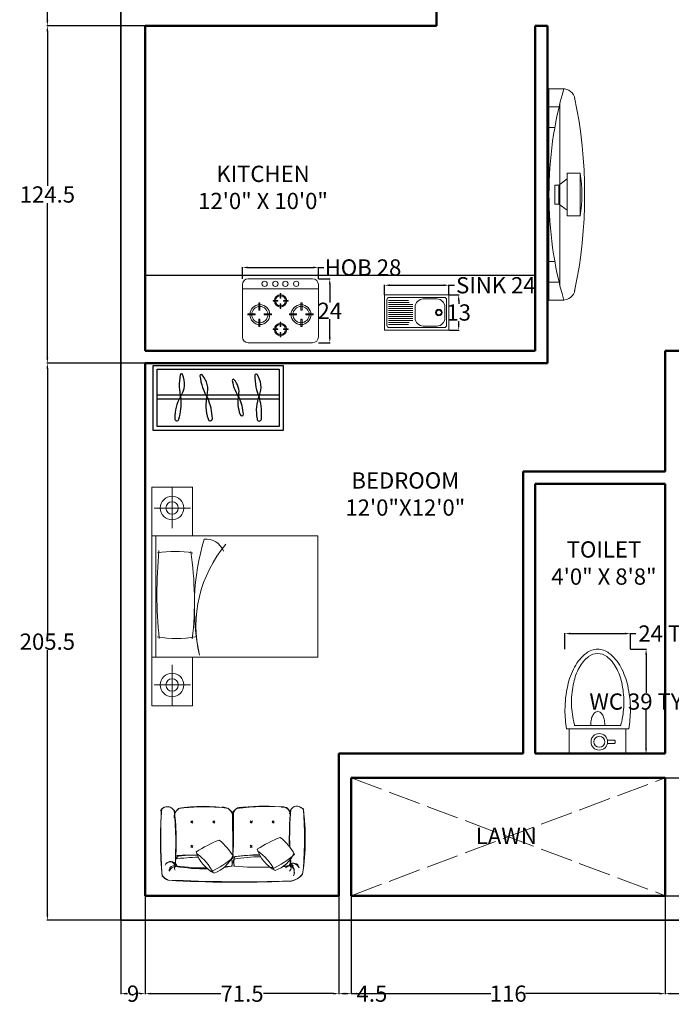
# Model space of a CAD drawing. Units: inches. Extents: x -20 to 10156, y 488 to 2970.
# Tile 1 of 6: x -20 to 221, y 488 to 851. Entities that reach past the tile are written whole.
import ezdxf

# ---------------------------------------------------------------- set-up
doc = ezdxf.new("R2010")
doc.units = ezdxf.units.IN
doc.header["$MEASUREMENT"] = 0
doc.linetypes.add('ACAD_ISO02W100', pattern=[15, 12, -3])
for name, color, linetype, lineweight in [('A-ANNO-DIMS', 2, 'Continuous', 18), ('A-AREA-IDEN', 7, 'Continuous', 25), ('A-EQPM', 9, 'Continuous', 18), ('A-FLOR-CASE', 8, 'Continuous', 25), ('A-FLOR-FIXT', 9, 'Continuous', 18), ('A-FURN', 8, 'Continuous', 18), ('A-WALL', 7, 'Continuous', 50), ('C-PROP', 7, 'Continuous', 35), ('L-PLNT-TURF', 8, 'ACAD_ISO02W100', 13)]:
    doc.layers.add(name, color=color, linetype=linetype, lineweight=lineweight)
doc.styles.get("Standard").update_dxf_attribs({"font": 'arial.ttf'})
doc.dimstyles.get("Standard").update_dxf_attribs({"dimtxt": 6, "dimasz": 2, "dimexe": 0.18, "dimexo": 0.0625, "dimgap": 0.09, "dimtad": 0, "dimtih": 1, "dimtoh": 1, "dimdec": 0, "dimzin": 0, "dimdsep": 46, "dimlunit": 4, "dimtxsty": 'Standard', "dimcen": 0.09, "dimadec": 0, "dimazin": 0, "dimtfac": 1, "dimtdec": 0, "dimtofl": 0, "dimtmove": 0, "dimatfit": 3, "dimfxl": 1, "dimtolj": 1, "dimtzin": 0, "dimarcsym": 0})

# ---------------------------------------------------------------- blocks, each defined once
blk = doc.blocks.new('A$C025C2FF6')
for p, q in [((45, 500), (550, 500)), ((0, 45), (0, 455)), ((241.9, 397.2), (241.9, 391.5)), ((277.6, 397.2), (241.9, 397.2)), ((241.9, 391.5), (277.6, 391.5)), ((277.6, 391.5), (277.6, 397.2)), ((295.2, 454.2), (300.9, 454.2)), ((295.2, 418.5), (295.2, 454.2)), ((300.9, 418.5), (295.2, 418.5)), ((300.9, 454.2), (300.9, 418.5)), ((322.1, 397.2), (357.7, 397.2)), ((322.1, 391.5), (322.1, 397.2)), ((357.7, 391.5), (322.1, 391.5)), ((357.7, 397.2), (357.7, 391.5)), ((595, 455), (595, 45)), ((128.2, 316.3), (128.2, 373.4)), ((128.2, 373.4), (137.4, 373.4)), ((137.4, 316.3), (128.2, 316.3)), ((137.4, 373.4), (137.4, 316.3)), ((295.2, 374), (295.2, 338.4)), ((300.9, 374), (295.2, 374)), ((295.2, 338.4), (300.9, 338.4)), ((300.9, 338.4), (300.9, 374)), ((467.8, 373.4), (458.7, 373.4)), ((458.7, 373.4), (458.7, 316.3)), ((458.7, 316.3), (467.8, 316.3)), ((467.8, 316.3), (467.8, 373.4)), ((100.1, 282.2), (43, 282.2)), ((43, 282.2), (43, 273.1)), ((43, 273.1), (100.1, 273.1)), ((100.1, 273.1), (100.1, 282.2)), ((128.2, 245.2), (128.2, 188.1)), ((137.4, 245.2), (128.2, 245.2)), ((137.4, 188.1), (137.4, 245.2)), ((171.3, 282.2), (228.3, 282.2)), ((171.3, 273.1), (171.3, 282.2)), ((228.3, 273.1), (171.3, 273.1)), ((228.3, 282.2), (228.3, 273.1)), ((367.8, 282.2), (367.8, 273.1)), ((424.8, 282.2), (367.8, 282.2)), ((367.8, 273.1), (424.8, 273.1)), ((424.8, 273.1), (424.8, 282.2)), ((458.7, 188.1), (458.7, 245.2)), ((458.7, 245.2), (467.8, 245.2)), ((467.8, 245.2), (467.8, 188.1)), ((496, 273.1), (496, 282.2)), ((496, 282.2), (553, 282.2)), ((553, 273.1), (496, 273.1)), ((553, 282.2), (553, 273.1)), ((128.2, 188.1), (137.4, 188.1)), ((277.6, 173.9), (241.9, 173.9)), ((241.9, 173.9), (241.9, 168.2)), ((241.9, 168.2), (277.6, 168.2)), ((277.6, 168.2), (277.6, 173.9)), ((295.2, 195.2), (295.2, 230.9)), ((295.2, 230.9), (300.9, 230.9)), ((300.9, 195.2), (295.2, 195.2)), ((300.9, 230.9), (300.9, 195.2)), ((322.1, 168.2), (322.1, 173.9)), ((322.1, 173.9), (357.7, 173.9)), ((357.7, 168.2), (322.1, 168.2)), ((357.7, 173.9), (357.7, 168.2)), ((467.8, 188.1), (458.7, 188.1)), ((300.9, 150.7), (295.2, 150.7)), ((295.2, 150.7), (295.2, 115.1)), ((295.2, 115.1), (300.9, 115.1)), ((300.9, 115.1), (300.9, 150.7)), ((1.2, 76.7), (594.9, 76.7)), ((550, 0), (45, 0))]:
    blk.add_line(p, q)
at = {"extrusion": (1e-16, 1e-16, -1)}
for centre, start_param, end_param in [((45, 455), 3.926991, 5.497787), ((550, 45), 0.785398, 2.356194)]:
    blk.add_ellipse(centre, major_axis=(31.8, 31.8), ratio=1, start_param=start_param, end_param=end_param, dxfattribs=at)
at = {"extrusion": (0, 0, -1)}
for centre, start_param, end_param in [((550, 455), 0.785398, 2.356194), ((45, 45), 3.926991, 5.497787)]:
    blk.add_ellipse(centre, major_axis=(-31.8, 31.8), ratio=1, start_param=start_param, end_param=end_param, dxfattribs=at)
at = {"extrusion": (1e-16, 3e-16, -1)}
for centre in [(298.7, 395.6), (298.7, 172.3)]:
    blk.add_ellipse(centre, major_axis=(-34.4, 34.4), ratio=1, start_param=5.497787, end_param=11.780972, dxfattribs=at)
at = {"extrusion": (1e-16, 2e-16, -1)}
for centre in [(298.7, 395.6), (298.7, 172.3)]:
    blk.add_ellipse(centre, major_axis=(-28.1, 28.1), ratio=1, start_param=5.497787, end_param=11.780972, dxfattribs=at)
at = {"extrusion": (-1e-16, -1e-16, -1)}
blk.add_ellipse((136.5, 279.7), major_axis=(-55.1, 55.1), ratio=1, start_param=5.497787, end_param=11.780972, dxfattribs=at)
at = {"extrusion": (0, -4e-16, -1)}
blk.add_ellipse((136.5, 279.7), major_axis=(-44.9, 44.9), ratio=1, start_param=5.497787, end_param=11.780972, dxfattribs=at)
for centre, major_axis, start_param, end_param in [((459.5, 279.7), (55.1, 55.1), 5.497787, 11.780972), ((459.5, 279.7), (44.9, 44.9), 5.497787, 11.780972), ((336.3, 39), (-14.8, 14.8), 3.926991, 10.210176), ((421.3, 39), (-14.8, 14.8), 3.926991, 10.210176)]:
    blk.add_ellipse(centre, major_axis=major_axis, ratio=1, start_param=start_param, end_param=end_param)
at = {"extrusion": (2e-16, -1e-16, -1)}
for centre in [(173.7, 39), (258.7, 39)]:
    blk.add_ellipse(centre, major_axis=(14.8, 14.8), ratio=1, start_param=3.926991, end_param=10.210176, dxfattribs=at)
blk = doc.blocks.new('A$C56104318')
for p, q in [((0, 0.609), (1.12, 0.609)), ((0, 0.609), (0, 0)), ((0.042, 0.525), (0.042, 0.084)), ((0.42, 0.515), (0.07, 0.515)), ((0.084, 0.567), (1.036, 0.567)), ((0.672, 0.539), (0.91, 0.539)), ((1.078, 0.525), (1.078, 0.084)), ((1.12, 0.609), (1.12, 0)), ((0.07, 0.48), (0.429, 0.48)), ((0.07, 0.445), (0.49, 0.445)), ((0.07, 0.41), (0.49, 0.41)), ((0.07, 0.375), (0.49, 0.375)), ((0.532, 0.21), (0.532, 0.399)), ((1.05, 0.399), (1.05, 0.21)), ((0.07, 0.34), (0.49, 0.34)), ((0.07, 0.305), (0.49, 0.305)), ((0.07, 0.27), (0.49, 0.27)), ((0.07, 0.235), (0.49, 0.235)), ((0.07, 0.2), (0.49, 0.2)), ((0.07, 0.165), (0.49, 0.165)), ((0.07, 0.13), (0.429, 0.13)), ((0.07, 0.094), (0.42, 0.094)), ((1.036, 0.042), (0.084, 0.042)), ((0.91, 0.07), (0.672, 0.07)), ((1.12, 0), (0, 0))]:
    blk.add_line(p, q)
for radius in [0.0574, 0.0427]:
    blk.add_circle((0.945, 0.305), radius)
for centre, radius, start, end in [((0.084, 0.525), 0.042, 90, 180), ((0.672, 0.399), 0.14, 90, 180), ((0.91, 0.399), 0.14, 0, 90), ((1.036, 0.525), 0.042, 0, 90), ((0.672, 0.21), 0.14, 180, 270), ((0.91, 0.21), 0.14, 270, 0), ((0.084, 0.084), 0.042, 180, 270), ((1.036, 0.084), 0.042, 270, 0)]:
    blk.add_arc(centre, radius, start, end)
blk = doc.blocks.new('A$C559B0E78')
at = {"xscale": 729, "yscale": 729, "zscale": 729}
blk.add_blockref('A$C56104318', (0, 0), dxfattribs=at)
blk = doc.blocks.new('A$C041817D3')
for p, q in [((0, 0), (0, 500)), ((0, 500), (1000, 500)), ((30, 30), (30, 470)), ((30, 470), (970, 470)), ((970, 470), (970, 30)), ((1000, 500), (1000, 0)), ((206.7, 270.8), (29.8, 270.8)), ((199, 240.8), (29.8, 240.8)), ((408.8, 240.8), (212.6, 240.8)), ((405.5, 270.8), (216.1, 270.8)), ((647.4, 270.8), (415.1, 270.8)), ((652.4, 240.8), (422, 240.8)), ((807.7, 270.8), (657.5, 270.8)), ((806.2, 240.8), (664.7, 240.8)), ((970.2, 270.8), (817, 270.8)), ((970.2, 240.8), (819.2, 240.8)), ((970, 30), (30, 30)), ((1000, 0), (0, 0))]:
    blk.add_line(p, q)
for centre, radius, start, end in [((621.4, 345.7), 421.4, 168.77299, 193.85802), ((217.3, 425.9), 9.38, 24.60956, 168.77299), ((72.1, 359.4), 169.1, 323.97798, 24.60956), ((368.6, 419.8), 9.38, 42.60956, 186.77299), ((777.7, 468.4), 421.4, 186.77299, 211.85802), ((251, 311.7), 169.1, 345.54145, 42.60956), ((615.5, 385.7), 7.5, 44.60956, 188.77299), ((941.3, 435.9), 337.1, 188.77299, 213.85802), ((524.6, 295.9), 135.3, 347.54145, 44.60956), ((791.5, 424.4), 9.38, 34.60956, 178.77299), ((1203.4, 415.6), 421.4, 178.77299, 203.85802), ((660.1, 333.7), 169.1, 337.54145, 34.60956), ((476.4, 102.2), 310, 149.58385, 181.67451), ((-230.1, 204), 444.3, 344.57561, 5.26247), ((715, 192.1), 310, 165.54145, 199.67451), ((11.6, 70.6), 444.3, 2.57561, 23.26247), ((898.8, 213.2), 248, 167.54145, 201.67451), ((339.9, 96.4), 355.4, 4.57561, 25.26247), ((1102.9, 150.7), 310, 157.54145, 191.67451), ((389.5, 128.2), 444.3, 354.57561, 15.26247), ((182.5, 90.2), 16.3, 169.40186, 344.57561), ((439.2, 89.8), 16.3, 187.40186, 2.57561), ((681.2, 123.8), 13, 189.40186, 4.57561), ((815.5, 87.8), 16.3, 179.40186, 354.57561)]:
    blk.add_arc(centre, radius, start, end)
blk = doc.blocks.new('A$C7FD35E1A')
for p, q in [((0.0233, 0.5799), (0.0233, 0.4408)), ((0.0233, 0.5799), (0.338, 0.5799)), ((0.338, 0.5799), (0.338, 0.4408)), ((0.2356, 0.5044), (0.275, 0.5044)), ((0.2357, 0.5217), (0.2745, 0.5217)), ((0.3542, 0.4408), (0.0087, 0.4408)), ((0.3093, 0.4224), (0.0536, 0.4224))]:
    blk.add_line(p, q)
for radius in [0.046, 0.0305]:
    blk.add_circle((0.1904, 0.5132), radius)
for centre, radius, start, end in [((0.2685, 0.5129), 0.0107, 307.488, 55.394), ((0.6238, 0.337), 0.6238, 170.4184, 180), ((-0.261, 0.337), 0.6238, 0, 9.5816), ((0.5354, 0.2931), 0.4991, 167.4267, 180), ((0.3603, 0.3321), 0.3197, 163.5954, 167.4267), ((0.277, 0.4171), 0.1337, 177.7133, 180), ((0.277, 0.4171), 0.1337, 180, 192.5399), ((0.23, 0.4066), 0.0855, 192.5399, 208.2349), ((0.1339, 0.4066), 0.0855, 331.7651, 347.4601), ((0.0869, 0.4171), 0.1337, 347.4601, 0), ((0.0869, 0.4171), 0.1337, 360, 2.2867), ((0.0026, 0.3321), 0.3197, 12.5733, 16.4046), ((-0.1725, 0.2931), 0.4991, 0, 12.5733), ((0.6238, 0.337), 0.6238, 180, 192.5733), ((0.2004, 0.3907), 0.052, 208.2349, 232.3543), ((0.182, 0.3668), 0.0218, 232.3543, 270), ((0.182, 0.3668), 0.0218, 270, 307.6457), ((0.1635, 0.3907), 0.052, 307.6457, 331.7651), ((-0.261, 0.337), 0.6238, 347.4267, 0), ((0.5354, 0.2931), 0.4991, 180, 192.5733), ((-0.1725, 0.2931), 0.4991, 347.4267, 0), ((0.405, 0.2881), 0.3996, 192.5733, 208.3008), ((0.3603, 0.254), 0.3197, 192.5733, 208.3008), ((0.0026, 0.254), 0.3197, 331.6992, 347.4267), ((-0.0421, 0.2881), 0.3996, 331.6992, 347.4267), ((0.2672, 0.214), 0.2432, 208.3008, 232.4306), ((0.2501, 0.1947), 0.1945, 208.3008, 232.4306), ((0.1128, 0.1947), 0.1945, 307.5694, 331.6992), ((0.0957, 0.214), 0.2432, 307.5694, 331.6992), ((0.1814, 0.1024), 0.1024, 232.4306, 270), ((0.1814, 0.1055), 0.082, 232.4306, 270), ((0.1814, 0.1055), 0.082, 270, 307.5694), ((0.1814, 0.1024), 0.1024, 270, 307.5694)]:
    blk.add_arc(centre, radius, start, end)
blk = doc.blocks.new('BED-WITH-NIGHTSTANDS')
for p, q in [((0, 80.86), (14.96, 80.86)), ((0, 62.91), (0, 80.86)), ((7.48, 73.12), (7.48, 80.95)), ((14.96, 80.86), (14.96, 62.91)), ((7.48, 73.12), (0.91, 73.12)), ((7.48, 73.12), (7.48, 65.64)), ((7.48, 73.12), (14.3, 73.12)), ((0, 62.91), (13.46, 62.91)), ((61.33, 62.91), (0, 62.91)), ((0, 18.04), (0, 62.91)), ((14.96, 62.91), (0, 62.91)), ((1.5, 18.04), (1.5, 62.91)), ((61.33, 18.04), (61.33, 62.91)), ((0, 18.04), (13.46, 18.04)), ((0, 18.04), (13.46, 18.04)), ((61.33, 18.04), (0, 18.04)), ((14.96, 18.04), (0, 18.04)), ((0, 18.04), (0, 0.09)), ((7.48, 7.83), (7.48, 15.31)), ((14.96, 0.09), (14.96, 18.04)), ((7.48, 7.83), (0.91, 7.83)), ((7.48, 7.83), (7.48, 0)), ((7.48, 7.83), (14.3, 7.83)), ((0, 0.09), (14.96, 0.09))]:
    blk.add_line(p, q)
for centre, radius in [((7.48, 73.12), 4.35), ((7.48, 73.12), 2.3), ((7.48, 7.83), 4.35), ((7.48, 7.83), 2.3)]:
    blk.add_circle(centre, radius)
for centre, radius, start, end in [((104.1, 36.77), 88.38, 163.6527, 191.7538), ((62.88, 29.59), 46.58, 139.6764, 193.4364), ((19.88, 54.53), 7.14, 22.4412, 94.6731), ((161.95, 41.88), 160.07, 174.4374, 186.047), ((8.44, 20.88), 36.25, 79.3149, 100.0855), ((-111.82, 38.85), 127.54, 353.7104, 8.2351), ((8.92, 63.63), 38.69, 259.7294, 280.8239)]:
    blk.add_arc(centre, radius, start, end)
blk = doc.blocks.new('*D14')
at = {"layer": 'A-ANNO-DIMS', "color": 0, "lineweight": -2, "transparency": 16777216}
for p, q in [((206, 618.67), (211.91, 618.67)), ((211.73, 616.67), (211.73, 602.56)), ((211.73, 582.06), (211.73, 596.17)), ((206, 580.06), (211.91, 580.06))]:
    blk.add_line(p, q, dxfattribs=at)
at = {"layer": 'A-ANNO-DIMS', "color": 0, "transparency": 16777216}
for points in [[(211.4, 616.67), (212.07, 616.67), (211.73, 618.67)], [(211.4, 582.06), (212.07, 582.06), (211.73, 580.06)]]:
    blk.add_solid(points, dxfattribs=at)
at = {"layer": 'Defpoints', "color": 0, "transparency": 16777216}
for p in [(205.94, 618.67), (205.94, 580.06), (211.73, 580.06)]:
    blk.add_point(p, dxfattribs=at)
at = {"layer": 'A-ANNO-DIMS', "color": 0, "transparency": 16777216, "insert": (211.73, 599.36), "char_height": 6, "attachment_point": 5}
blk.add_mtext('\\A1;WC 39 TYP.', dxfattribs=at)
blk = doc.blocks.new('*D15')
at = {"layer": 'A-ANNO-DIMS', "color": 0, "lineweight": -2, "transparency": 16777216}
for p, q in [((181.78, 618.73), (181.78, 624.64)), ((183.78, 624.46), (203.94, 624.46)), ((205.94, 618.73), (205.94, 624.64)), ((205.94, 624.46), (207.94, 624.46))]:
    blk.add_line(p, q, dxfattribs=at)
at = {"layer": 'A-ANNO-DIMS', "color": 0, "transparency": 16777216}
for points in [[(183.78, 624.79), (183.78, 624.13), (181.78, 624.46)], [(203.94, 624.79), (203.94, 624.13), (205.94, 624.46)]]:
    blk.add_solid(points, dxfattribs=at)
at = {"layer": 'Defpoints', "color": 0, "transparency": 16777216}
for p in [(205.94, 624.46), (181.78, 618.67), (205.94, 618.67)]:
    blk.add_point(p, dxfattribs=at)
at = {"layer": 'A-ANNO-DIMS', "color": 0, "transparency": 16777216, "insert": (222.69, 624.46), "char_height": 6, "attachment_point": 5}
blk.add_mtext('\\A1;24 TYP.', dxfattribs=at)
blk = doc.blocks.new('*D24')
at = {"layer": 'A-ANNO-DIMS', "color": 0, "lineweight": -2, "transparency": 16777216}
for p, q in [((62.67, 755.4), (62.67, 759.72)), ((64.67, 759.54), (88.72, 759.54)), ((90.72, 755.4), (90.72, 759.72)), ((90.72, 759.54), (92.72, 759.54))]:
    blk.add_line(p, q, dxfattribs=at)
at = {"layer": 'A-ANNO-DIMS', "color": 0, "transparency": 16777216}
for points in [[(64.67, 759.88), (64.67, 759.21), (62.67, 759.54)], [(88.72, 759.88), (88.72, 759.21), (90.72, 759.54)]]:
    blk.add_solid(points, dxfattribs=at)
at = {"layer": 'Defpoints', "color": 0, "transparency": 16777216}
for p in [(90.72, 759.54), (62.67, 755.34), (90.72, 755.34)]:
    blk.add_point(p, dxfattribs=at)
at = {"layer": 'A-ANNO-DIMS', "color": 0, "transparency": 16777216, "insert": (107.2, 759.54), "char_height": 6, "attachment_point": 5}
blk.add_mtext('\\A1;HOB 28', dxfattribs=at)
blk = doc.blocks.new('*D25')
at = {"layer": 'A-ANNO-DIMS', "color": 0, "lineweight": -2, "transparency": 16777216}
for p, q in [((90.78, 755.34), (95.11, 755.34)), ((94.93, 753.34), (94.93, 746.65)), ((94.93, 733.76), (94.93, 740.45)), ((90.78, 731.76), (95.11, 731.76))]:
    blk.add_line(p, q, dxfattribs=at)
at = {"layer": 'A-ANNO-DIMS', "color": 0, "transparency": 16777216}
for points in [[(94.6, 753.34), (95.26, 753.34), (94.93, 755.34)], [(94.6, 733.76), (95.26, 733.76), (94.93, 731.76)]]:
    blk.add_solid(points, dxfattribs=at)
at = {"layer": 'Defpoints', "color": 0, "transparency": 16777216}
for p in [(90.72, 755.34), (90.72, 731.76), (94.93, 731.76)]:
    blk.add_point(p, dxfattribs=at)
at = {"layer": 'A-ANNO-DIMS', "color": 0, "transparency": 16777216, "insert": (94.93, 743.55), "char_height": 6, "attachment_point": 5}
blk.add_mtext('\\A1;24', dxfattribs=at)
blk = doc.blocks.new('*D26')
at = {"layer": 'A-ANNO-DIMS', "color": 0, "lineweight": -2, "transparency": 16777216}
for p, q in [((115.12, 749.47), (115.12, 753.17)), ((117.12, 752.99), (136.95, 752.99)), ((138.95, 749.47), (138.95, 753.17)), ((138.95, 752.99), (140.95, 752.99))]:
    blk.add_line(p, q, dxfattribs=at)
at = {"layer": 'A-ANNO-DIMS', "color": 0, "transparency": 16777216}
for points in [[(117.12, 753.32), (117.12, 752.65), (115.12, 752.99)], [(136.95, 753.32), (136.95, 752.65), (138.95, 752.99)]]:
    blk.add_solid(points, dxfattribs=at)
at = {"layer": 'Defpoints', "color": 0, "transparency": 16777216}
for p in [(138.95, 752.99), (115.12, 749.41), (138.95, 749.41)]:
    blk.add_point(p, dxfattribs=at)
at = {"layer": 'A-ANNO-DIMS', "color": 0, "transparency": 16777216, "insert": (156.26, 752.99), "char_height": 6, "attachment_point": 5}
blk.add_mtext('\\A1;SINK 24', dxfattribs=at)
blk = doc.blocks.new('*D27')
at = {"layer": 'A-ANNO-DIMS', "color": 0, "lineweight": -2, "transparency": 16777216}
for p, q in [((139.02, 749.41), (142.71, 749.41)), ((142.53, 747.41), (142.53, 746.09)), ((142.53, 738.45), (142.53, 739.77)), ((139.02, 736.45), (142.71, 736.45))]:
    blk.add_line(p, q, dxfattribs=at)
at = {"layer": 'A-ANNO-DIMS', "color": 0, "transparency": 16777216}
for points in [[(142.2, 747.41), (142.86, 747.41), (142.53, 749.41)], [(142.2, 738.45), (142.86, 738.45), (142.53, 736.45)]]:
    blk.add_solid(points, dxfattribs=at)
at = {"layer": 'Defpoints', "color": 0, "transparency": 16777216}
for p in [(138.95, 749.41), (138.95, 736.45), (142.53, 736.45)]:
    blk.add_point(p, dxfattribs=at)
at = {"layer": 'A-ANNO-DIMS', "color": 0, "transparency": 16777216, "insert": (142.53, 742.93), "char_height": 6, "attachment_point": 5}
blk.add_mtext('\\A1;13', dxfattribs=at)
blk = doc.blocks.new('*D32')
at = {"layer": 'A-ANNO-DIMS', "color": 0, "lineweight": -2, "transparency": 16777216}
for p, q in [((26.74, 917.23), (-9.53, 917.23)), ((-9.35, 915.23), (-9.35, 886.13)), ((-9.35, 850.73), (-9.35, 879.83)), ((26.74, 848.73), (-9.53, 848.73))]:
    blk.add_line(p, q, dxfattribs=at)
at = {"layer": 'A-ANNO-DIMS', "color": 0, "transparency": 16777216}
for points in [[(-9.68, 915.23), (-9.02, 915.23), (-9.35, 917.23)], [(-9.68, 850.73), (-9.02, 850.73), (-9.35, 848.73)]]:
    blk.add_solid(points, dxfattribs=at)
at = {"layer": 'Defpoints', "color": 0, "transparency": 16777216}
for p in [(26.8, 917.23), (-9.35, 848.73), (26.8, 848.73)]:
    blk.add_point(p, dxfattribs=at)
at = {"layer": 'A-ANNO-DIMS', "color": 0, "transparency": 16777216, "insert": (-9.35, 882.98), "char_height": 6, "attachment_point": 5}
blk.add_mtext('\\A1;68.5', dxfattribs=at)
blk = doc.blocks.new('*D33')
at = {"layer": 'A-ANNO-DIMS', "color": 0, "lineweight": -2, "transparency": 16777216}
for p, q in [((26.74, 848.73), (-9.53, 848.73)), ((-9.35, 846.73), (-9.35, 789.63)), ((-9.35, 726.23), (-9.35, 783.33)), ((26.74, 724.23), (-9.53, 724.23))]:
    blk.add_line(p, q, dxfattribs=at)
at = {"layer": 'A-ANNO-DIMS', "color": 0, "transparency": 16777216}
for points in [[(-9.68, 846.73), (-9.02, 846.73), (-9.35, 848.73)], [(-9.68, 726.23), (-9.02, 726.23), (-9.35, 724.23)]]:
    blk.add_solid(points, dxfattribs=at)
at = {"layer": 'Defpoints', "color": 0, "transparency": 16777216}
for p in [(26.8, 848.73), (-9.35, 724.23), (26.8, 724.23)]:
    blk.add_point(p, dxfattribs=at)
at = {"layer": 'A-ANNO-DIMS', "color": 0, "transparency": 16777216, "insert": (-9.35, 786.48), "char_height": 6, "attachment_point": 5}
blk.add_mtext('\\A1;124.5', dxfattribs=at)
blk = doc.blocks.new('*D34')
at = {"layer": 'A-ANNO-DIMS', "color": 0, "lineweight": -2, "transparency": 16777216}
for p, q in [((26.74, 724.23), (-9.53, 724.23)), ((-9.35, 722.23), (-9.35, 624.63)), ((-9.35, 520.73), (-9.35, 618.33)), ((17.74, 518.73), (-9.53, 518.73))]:
    blk.add_line(p, q, dxfattribs=at)
at = {"layer": 'A-ANNO-DIMS', "color": 0, "transparency": 16777216}
for points in [[(-9.68, 722.23), (-9.02, 722.23), (-9.35, 724.23)], [(-9.68, 520.73), (-9.02, 520.73), (-9.35, 518.73)]]:
    blk.add_solid(points, dxfattribs=at)
at = {"layer": 'Defpoints', "color": 0, "transparency": 16777216}
for p in [(26.8, 724.23), (-9.35, 518.73), (17.8, 518.73)]:
    blk.add_point(p, dxfattribs=at)
at = {"layer": 'A-ANNO-DIMS', "color": 0, "transparency": 16777216, "insert": (-9.35, 621.48), "char_height": 6, "attachment_point": 5}
blk.add_mtext('\\A1;205.5', dxfattribs=at)
blk = doc.blocks.new('*D35')
at = {"layer": 'A-ANNO-DIMS', "color": 0, "lineweight": -2, "transparency": 16777216}
for p, q in [((26.8, 527.67), (26.8, 491.4)), ((17.8, 518.67), (17.8, 491.4)), ((19.8, 491.58), (20.24, 491.58)), ((24.8, 491.58), (24.36, 491.58))]:
    blk.add_line(p, q, dxfattribs=at)
at = {"layer": 'A-ANNO-DIMS', "color": 0, "transparency": 16777216}
for points in [[(19.8, 491.91), (19.8, 491.25), (17.8, 491.58)], [(24.8, 491.91), (24.8, 491.25), (26.8, 491.58)]]:
    blk.add_solid(points, dxfattribs=at)
at = {"layer": 'Defpoints', "color": 0, "transparency": 16777216}
for p in [(26.8, 527.73), (17.8, 518.73), (26.8, 491.58)]:
    blk.add_point(p, dxfattribs=at)
at = {"layer": 'A-ANNO-DIMS', "color": 0, "transparency": 16777216, "insert": (22.3, 491.58), "char_height": 6, "attachment_point": 5}
blk.add_mtext('\\A1;9', dxfattribs=at)
blk = doc.blocks.new('*D36')
at = {"layer": 'A-ANNO-DIMS', "color": 0, "lineweight": -2, "transparency": 16777216}
for p, q in [((26.8, 527.67), (26.8, 491.4)), ((98.3, 527.67), (98.3, 491.4)), ((28.8, 491.58), (54.67, 491.58)), ((96.3, 491.58), (70.43, 491.58))]:
    blk.add_line(p, q, dxfattribs=at)
at = {"layer": 'A-ANNO-DIMS', "color": 0, "transparency": 16777216}
for points in [[(28.8, 491.91), (28.8, 491.25), (26.8, 491.58)], [(96.3, 491.91), (96.3, 491.25), (98.3, 491.58)]]:
    blk.add_solid(points, dxfattribs=at)
at = {"layer": 'Defpoints', "color": 0, "transparency": 16777216}
for p in [(26.8, 527.73), (98.3, 527.73), (98.3, 491.58)]:
    blk.add_point(p, dxfattribs=at)
at = {"layer": 'A-ANNO-DIMS', "color": 0, "transparency": 16777216, "insert": (62.55, 491.58), "char_height": 6, "attachment_point": 5}
blk.add_mtext('\\A1;71.5', dxfattribs=at)
blk = doc.blocks.new('*D37')
at = {"layer": 'A-ANNO-DIMS', "color": 0, "lineweight": -2, "transparency": 16777216}
for p, q in [((98.3, 527.67), (98.3, 491.4)), ((102.8, 527.67), (102.8, 491.4)), ((100.3, 491.58), (100.8, 491.58)), ((102.8, 491.58), (104.8, 491.58))]:
    blk.add_line(p, q, dxfattribs=at)
at = {"layer": 'A-ANNO-DIMS', "color": 0, "transparency": 16777216}
for points in [[(100.3, 491.91), (100.3, 491.25), (98.3, 491.58)], [(100.8, 491.91), (100.8, 491.25), (102.8, 491.58)]]:
    blk.add_solid(points, dxfattribs=at)
at = {"layer": 'Defpoints', "color": 0, "transparency": 16777216}
for p in [(98.3, 527.73), (102.8, 527.73), (102.8, 491.58)]:
    blk.add_point(p, dxfattribs=at)
at = {"layer": 'A-ANNO-DIMS', "color": 0, "transparency": 16777216, "insert": (110.49, 491.58), "char_height": 6, "attachment_point": 5}
blk.add_mtext('\\A1;4.5', dxfattribs=at)
blk = doc.blocks.new('*D38')
at = {"layer": 'A-ANNO-DIMS', "color": 0, "lineweight": -2, "transparency": 16777216}
for p, q in [((102.8, 527.67), (102.8, 491.4)), ((218.8, 527.67), (218.8, 491.4)), ((104.8, 491.58), (154.37, 491.58)), ((216.8, 491.58), (167.23, 491.58))]:
    blk.add_line(p, q, dxfattribs=at)
at = {"layer": 'A-ANNO-DIMS', "color": 0, "transparency": 16777216}
for points in [[(104.8, 491.91), (104.8, 491.25), (102.8, 491.58)], [(216.8, 491.91), (216.8, 491.25), (218.8, 491.58)]]:
    blk.add_solid(points, dxfattribs=at)
at = {"layer": 'Defpoints', "color": 0, "transparency": 16777216}
for p in [(102.8, 527.73), (218.8, 527.73), (218.8, 491.58)]:
    blk.add_point(p, dxfattribs=at)
at = {"layer": 'A-ANNO-DIMS', "color": 0, "transparency": 16777216, "insert": (160.8, 491.58), "char_height": 6, "attachment_point": 5}
blk.add_mtext('\\A1;116', dxfattribs=at)
blk = doc.blocks.new('*D39')
at = {"layer": 'A-ANNO-DIMS', "color": 0, "lineweight": -2, "transparency": 16777216}
for p, q in [((218.8, 527.67), (218.8, 491.4)), ((377.8, 518.67), (377.8, 491.4)), ((220.8, 491.58), (291.86, 491.58)), ((375.8, 491.58), (304.74, 491.58))]:
    blk.add_line(p, q, dxfattribs=at)
at = {"layer": 'A-ANNO-DIMS', "color": 0, "transparency": 16777216}
for points in [[(220.8, 491.91), (220.8, 491.25), (218.8, 491.58)], [(375.8, 491.91), (375.8, 491.25), (377.8, 491.58)]]:
    blk.add_solid(points, dxfattribs=at)
at = {"layer": 'Defpoints', "color": 0, "transparency": 16777216}
for p in [(218.8, 527.73), (377.8, 518.73), (377.8, 491.58)]:
    blk.add_point(p, dxfattribs=at)
at = {"layer": 'A-ANNO-DIMS', "color": 0, "transparency": 16777216, "insert": (298.3, 491.58), "char_height": 6, "attachment_point": 5}
blk.add_mtext('\\A1;159', dxfattribs=at)
blk = doc.blocks.new('*D40')
at = {"layer": 'A-ANNO-DIMS', "color": 0, "lineweight": -2, "transparency": 16777216}
for p, q in [((218.86, 571.23), (246.13, 571.23)), ((245.95, 569.23), (245.95, 552.64)), ((245.95, 529.73), (245.95, 546.32)), ((218.86, 527.73), (246.13, 527.73))]:
    blk.add_line(p, q, dxfattribs=at)
at = {"layer": 'A-ANNO-DIMS', "color": 0, "transparency": 16777216}
for points in [[(245.62, 569.23), (246.28, 569.23), (245.95, 571.23)], [(245.62, 529.73), (246.28, 529.73), (245.95, 527.73)]]:
    blk.add_solid(points, dxfattribs=at)
at = {"layer": 'Defpoints', "color": 0, "transparency": 16777216}
for p in [(218.8, 571.23), (218.8, 527.73), (245.95, 527.73)]:
    blk.add_point(p, dxfattribs=at)
at = {"layer": 'A-ANNO-DIMS', "color": 0, "transparency": 16777216, "insert": (245.95, 549.48), "char_height": 6, "attachment_point": 5}
blk.add_mtext('\\A1;43.5', dxfattribs=at)

msp = doc.modelspace()

# ---------------------------------------------------------------- linework, layer by layer
at = {"layer": 'A-EQPM'}
for p, q in [((175.86, 747.52), (175.86, 825.47)), ((181.35, 825.47), (175.86, 825.47)), ((181.35, 825.47), (181.39, 825.47)), ((175.86, 818.88), (179.63, 818.88)), ((179.9, 819.98), (179.9, 753.01)), ((175.86, 811.2), (178.04, 811.2)), ((182.59, 792.2), (179.55, 789.95)), ((182.59, 794.37), (187.37, 794.37)), ((182.59, 794.37), (182.59, 778.54)), ((187.37, 794.37), (187.37, 778.54)), ((178.01, 782.95), (178.01, 789.95)), ((179.55, 789.95), (178.01, 789.95)), ((179.55, 782.95), (179.55, 789.95)), ((179.55, 782.95), (178.01, 782.95)), ((182.59, 780.71), (179.55, 782.95)), ((182.59, 778.54), (187.37, 778.54)), ((175.86, 761.79), (178.04, 761.79)), ((175.86, 754.11), (179.63, 754.11)), ((175.86, 747.52), (181.35, 747.52)), ((181.35, 747.52), (181.39, 747.52))]:
    msp.add_line(p, q, dxfattribs=at)
msp.add_lwpolyline([(185.35, 822.22, -0.103184), (185.35, 750.77, -0.103184)], format="xyb", dxfattribs=at)
for centre, radius, start, end in [((316.97, 786.49), 141.11, 163.9658, 196.0342), ((181.11, 821.09), 4.39, 8.4687, 93.693), ((139.09, 786.45), 48.93, 350.6925, 9.3075), ((181.11, 751.9), 4.39, 266.307, 351.5313)]:
    msp.add_arc(centre, radius, start, end, dxfattribs=at)
at = {"layer": 'A-FLOR-CASE'}
msp.add_line((26.8, 756.73), (170.8, 756.73), dxfattribs=at)
at = {"layer": 'A-FURN'}
for p, q in [((44.41, 555.29), (43.65, 554.55)), ((43.66, 555.3), (44.4, 554.54)), ((52.51, 555.29), (51.75, 554.55)), ((51.76, 555.3), (52.5, 554.54)), ((66.34, 555.29), (65.58, 554.55)), ((65.59, 555.3), (66.33, 554.54)), ((74.43, 555.29), (73.67, 554.55)), ((73.68, 555.3), (74.42, 554.54)), ((44.37, 546.3), (43.61, 545.55)), ((43.62, 546.31), (44.36, 545.55)), ((66.3, 546.3), (65.54, 545.55)), ((65.55, 546.31), (66.29, 545.55))]:
    msp.add_line(p, q, dxfattribs=at)
for centre, radius, start, end in [((34.94, 557.78), 2.83, 14.6379, 154.3095), ((176.69, 548.41), 144.28, 175.4325, 185.431), ((244.3, 549.68), 211.76, 177.3143, 183.933), ((34.94, 557.51), 3.02, 33.041, 136.0653), ((40.96, 556.8), 3.46, 100.9756, 184.9747), ((40.86, 557.12), 3.21, 109.8228, 182.4985), ((48.43, 508), 52.71, 80.0543, 100.4167), ((48.36, 490.17), 70.37, 85.2072, 97.551), ((55.21, 556.24), 4.17, 6.5867, 103.4511), ((55.99, 557.2), 3.04, 354.9234, 65.6374), ((61.7, 557.45), 2.67, 73.4437, 181.8228), ((62.03, 557.65), 2.69, 72.9316, 185.1092), ((71.72, 477.07), 83.56, 84.8245, 97.7148), ((70.42, 490.01), 70.76, 85.0781, 97.695), ((77.24, 557.53), 3.07, 357.6579, 104.0974), ((78.02, 558.3), 2.13, 350.2617, 111.0115), ((222.96, 549.09), 142.84, 175.8027, 181.3803), ((82.84, 558.16), 2.64, 17.7157, 162.8428), ((82.61, 557.55), 3.19, 36.0678, 112.6723), ((6.39, 548.49), 79.5, 350.8079, 8.3514), ((-44.25, 547.69), 82.52, 352.9836, 7.989), ((-146.93, 546.47), 184.97, 357.5073, 3.9592), ((1409381.54, 25679.21), 1409546.47, 181.02115803, 181.02184547), ((-64.17, 551.5), 123.6, 355.8425, 3.2873), ((197.5, 548.58), 117.52, 174.7422, 181.3335), ((-43.61, 549.01), 129.21, 354.0627, 4.6253), ((94.67, 503.15), 49.47, 111.3371, 122.4176), ((61.98, 531.37), 23.12, 30.3068, 50.5663), ((72.12, 502.18), 49.47, 111.3371, 122.4176), ((39.43, 530.4), 23.12, 30.3068, 50.5663), ((48.33, 460.87), 81.09, 91.3731, 97.4472), ((40.27, 540.28), 2.35, 96.1174, 223.1189), ((39.82, 540.61), 1.87, 77.6226, 170.3094), ((45.17, 404.68), 138.03, 89.6386, 92.7653), ((47.47, 431.76), 111, 90.7456, 94.456), ((58.23, 547.8), 13.21, 197.0126, 242.9429), ((35.76, 528.42), 17.88, 25.9005, 55.6513), ((38.39, 565.17), 31.22, 294.0815, 312.2768), ((48.29, 547.16), 11.79, 289.4501, 336.7699), ((-64.17, 551.5), 123.6, 355.3655, 355.4784), ((57.79, 540.63), 1.68, 29.1313, 42.0141), ((70.98, 472.11), 70.81, 91.6458, 99.5268), ((51.49, 569.2), 28.33, 285.9625, 287.4638), ((45.17, 404.68), 138.03, 83.8872, 84.1215), ((70.54, 475.8), 66.32, 91.0061, 99.6001), ((66.1, 540.29), 6.6, 164.0479, 194.2061), ((69.81, 453.69), 89.04, 90.4949, 96.3291), ((80.78, 548.77), 13.21, 197.0126, 242.9429), ((58.31, 529.39), 17.88, 25.9005, 55.6513), ((60.94, 566.14), 31.22, 294.0815, 312.2768), ((70.85, 548.12), 11.79, 289.4501, 336.7699), ((36.19, 538.1), 2.25, 42.3134, 157.6102), ((35.96, 538.2), 2.01, 14.7814, 157.5922), ((37.43, 537.04), 1.77, 88.0108, 186.5585), ((38.16, 535.82), 2.68, 91.184, 157.8216), ((39.11, 537.98), 1.52, 134.3938, 213.5856), ((48.14, 595.29), 57.63, 259.9466, 271.5903), ((48.67, 612.12), 74.14, 262.1551, 270.5585), ((48.14, 595.29), 57.63, 277.803, 280.4557), ((48.67, 612.12), 74.14, 275.7795, 278.522), ((48.33, 460.87), 81.09, 82.7245, 82.7726), ((54.97, 539.79), 3.94, 343.3108, 22.6164), ((56.3, 539.99), 2.67, 329.8319, 29.468), ((64.85, 540.39), 5.43, 171.5362, 198.3493), ((69.19, 634.88), 96.68, 264.3639, 272.1219), ((69.93, 618.23), 80.2, 272.2017, 272.8482), ((69.93, 618.23), 80.2, 275.4058, 278.3067), ((69.19, 634.88), 96.68, 275.0871, 276.7491), ((78.12, 540.28), 2.26, 280.6216, 19.193), ((78.88, 536.33), 2.98, 334.8715, 66.7247), ((81.59, 537.73), 2.01, 9.2916, 137.6289), ((78.35, 538.38), 2.38, 317.7203, 24.4461), ((78.49, 540.4), 2.03, 327.7366, 22.2387), ((197.5, 548.58), 117.52, 183.7101, 185.0653), ((80.86, 536.63), 3.07, 27.8433, 99.8684), ((222.96, 549.09), 142.84, 183.1908, 183.7892), ((77.12, 536.58), 4.7, 341.2473, 41.1348), ((36.46, 537.29), 4.04, 211.8817, 253.9672), ((38.84, 540.65), 8.02, 223.5462, 243.1435), ((79.69, 539.29), 6.25, 263.8792, 327.1093), ((79.17, 540.69), 7.65, 278.6549, 318.7104), ((62.47, 1104.91), 572.05, 267.2697, 271.7875), ((60.53, 968.43), 435.75, 266.6876, 272.4329)]:
    msp.add_arc(centre, radius, start, end, dxfattribs=at)
at = {"layer": 'A-WALL'}
for p, q in [((134.3, 917.23), (134.3, 848.73)), ((26.8, 848.73), (134.3, 848.73)), ((26.8, 728.73), (26.8, 848.73)), ((170.8, 728.73), (170.8, 848.73)), ((170.8, 848.73), (175.3, 848.73)), ((175.3, 724.23), (175.3, 848.73)), ((26.8, 728.73), (170.8, 728.73)), ((218.8, 728.73), (368.8, 728.73)), ((218.8, 684.23), (218.8, 728.73)), ((26.8, 527.73), (26.8, 724.23)), ((26.8, 724.23), (175.3, 724.23)), ((166.3, 580.23), (166.3, 684.23)), ((166.3, 684.23), (218.8, 684.23)), ((170.8, 580.23), (170.8, 679.73)), ((170.8, 679.73), (218.8, 679.73)), ((218.8, 580.23), (218.8, 679.73)), ((98.3, 580.23), (166.3, 580.23)), ((98.3, 527.73), (98.3, 580.23)), ((170.8, 580.23), (218.8, 580.23)), ((102.8, 571.23), (218.8, 571.23)), ((102.8, 527.73), (102.8, 571.23)), ((218.8, 527.73), (218.8, 571.23)), ((98.3, 527.73), (26.8, 527.73)), ((218.8, 527.73), (102.8, 527.73))]:
    msp.add_line(p, q, dxfattribs=at)
at = {"layer": 'C-PROP'}
for p, q in [((17.8, 518.73), (17.8, 1058.73)), ((377.8, 518.73), (17.8, 518.73))]:
    msp.add_line(p, q, dxfattribs=at)
at = {"layer": 'L-PLNT-TURF'}
for p, q in [((102.8, 527.73), (218.8, 571.23)), ((102.8, 571.23), (218.8, 527.73))]:
    msp.add_line(p, q, dxfattribs=at)

# ---------------------------------------------------------------- block references
at = {"layer": 'A-EQPM', "xscale": -0.0471474330273417, "yscale": 0.0471474330273417, "zscale": 0.0471474330273417, "rotation": 180}
msp.add_blockref('A$C025C2FF6', (62.67, 755.34), dxfattribs=at)
at = {"layer": 'A-FLOR-CASE', "xscale": 0.048, "yscale": 0.048, "zscale": 0.048}
msp.add_blockref('A$C041817D3', (29.74, 699.43), dxfattribs=at)
at = {"layer": 'A-FLOR-FIXT', "rotation": 180}
for name, p, xscale, yscale, zscale in [('A$C559B0E78', (115.12, 749.41), -0.0291919031128754, 0.0291919031128754, 0.0291919031128754), ('A$C7FD35E1A', (181.78, 618.67), -66.57190006508344, 66.57190006508344, 66.57190006508344)]:
    msp.add_blockref(name, p, dxfattribs=dict(at, xscale=xscale, yscale=yscale, zscale=zscale))
at = {"layer": 'A-FURN'}
msp.add_blockref('BED-WITH-NIGHTSTANDS', (29.22, 597.66), dxfattribs=at)

# ---------------------------------------------------------------- texts
at = {"layer": 'A-AREA-IDEN', "char_height": 6, "attachment_point": 1}
for s, width, insert in [('\\pxqc;KITCHEN\\P12\'0" X 10\'0"', 80.4728, (30.04, 797.09)), ('\\pxqc;BEDROOM\\P12\'0"X12\'0"', 105.4912, (70.07, 683.95)), ('\\pxqc;TOILET\\P4\'0" X 8\'8"', 68.8926, (161.73, 658.49)), ('LAWN', 71.0846, (148.85, 552.78))]:
    msp.add_mtext_dynamic_manual_height_columns(s, width=width, gutter_width=30, heights=[0], dxfattribs=dict(at, insert=insert))

# ---------------------------------------------------------------- dimensions: what is measured, and where the dimension line sits
at = {"layer": 'A-ANNO-DIMS'}
for base, p1, p2, angle, override, picture, middle in [((-9.35, 848.73), (26.8, 917.23), (26.8, 848.73), 90, {"dimdec": 1, "dimlfac": 1, "dimrnd": 0, "dimzin": 0, "dimdsep": 46, "dimlunit": 2}, '*D32', (-9.35, 882.98)), ((-9.35, 724.23), (26.8, 848.73), (26.8, 724.23), 90, {"dimdec": 1, "dimlfac": 1, "dimrnd": 0, "dimzin": 0, "dimdsep": 46, "dimlunit": 2}, '*D33', (-9.35, 786.48)), ((94.93, 731.76), (90.72, 755.34), (90.72, 731.76), 270, {"dimdec": 0, "dimlfac": 1, "dimrnd": 0, "dimzin": 0, "dimdsep": 46, "dimlunit": 2}, '*D25', (94.93, 743.55)), ((142.53, 736.45), (138.95, 749.41), (138.95, 736.45), 270, {"dimdec": 0, "dimlfac": 1, "dimrnd": 0, "dimzin": 0, "dimdsep": 46, "dimlunit": 2}, '*D27', (142.53, 742.93)), ((-9.35, 518.73), (26.8, 724.23), (17.8, 518.73), 90, {"dimdec": 1, "dimlfac": 1, "dimrnd": 0, "dimzin": 0, "dimdsep": 46, "dimlunit": 2}, '*D34', (-9.35, 621.48)), ((245.95, 527.73), (218.8, 571.23), (218.8, 527.73), 270, {"dimdec": 1, "dimlfac": 1, "dimrnd": 0, "dimzin": 0, "dimdsep": 46, "dimlunit": 2}, '*D40', (245.95, 549.48))]:
    dim = msp.add_linear_dim(base=base, p1=p1, p2=p2, angle=angle, dimstyle='Standard', override=override, dxfattribs=at)
    dim.commit()
    dim.dimension.update_dxf_attribs({"geometry": picture, "text_midpoint": middle})
for base, p1, p2, text, picture, middle in [((90.72, 759.54), (62.67, 755.34), (90.72, 755.34), 'HOB <>', '*D24', (107.2, 759.54)), ((138.95, 752.99), (115.12, 749.41), (138.95, 749.41), 'SINK <>', '*D26', (156.26, 752.99)), ((205.94, 624.46), (181.78, 618.67), (205.94, 618.67), '<> TYP.', '*D15', (222.69, 624.46))]:
    dim = msp.add_linear_dim(base=base, p1=p1, p2=p2, text=text, dimstyle='Standard', override={"dimdec": 0, "dimlfac": 1, "dimrnd": 0, "dimzin": 0, "dimdsep": 46, "dimlunit": 2}, dxfattribs=at)
    dim.commit()
    dim.dimension.update_dxf_attribs({"geometry": picture, "text_midpoint": middle})
dim = msp.add_linear_dim(base=(211.73, 580.06), p1=(205.94, 618.67), p2=(205.94, 580.06), angle=270, text='WC <> TYP.', dimstyle='Standard', override={"dimdec": 0, "dimlfac": 1, "dimrnd": 0, "dimzin": 0, "dimdsep": 46, "dimlunit": 2}, dxfattribs=at)
dim.commit()
dim.dimension.update_dxf_attribs({"geometry": '*D14', "text_midpoint": (211.73, 599.36)})
for base, p1, p2, override, picture, middle in [((26.8, 491.58), (17.8, 518.73), (26.8, 527.73), {"dimdec": 0, "dimlfac": 1, "dimrnd": 0, "dimzin": 0, "dimdsep": 46, "dimlunit": 2}, '*D35', (22.3, 491.58)), ((98.3, 491.58), (26.8, 527.73), (98.3, 527.73), {"dimdec": 1, "dimlfac": 1, "dimrnd": 0, "dimzin": 0, "dimdsep": 46, "dimlunit": 2}, '*D36', (62.55, 491.58)), ((102.8, 491.58), (98.3, 527.73), (102.8, 527.73), {"dimdec": 1, "dimlfac": 1, "dimrnd": 0, "dimzin": 0, "dimdsep": 46, "dimlunit": 2}, '*D37', (110.49, 491.58)), ((218.8, 491.58), (102.8, 527.73), (218.8, 527.73), {"dimdec": 0, "dimlfac": 1, "dimrnd": 0, "dimzin": 0, "dimdsep": 46, "dimlunit": 2}, '*D38', (160.8, 491.58)), ((377.8, 491.58), (218.8, 527.73), (377.8, 518.73), {"dimdec": 0, "dimlfac": 1, "dimrnd": 0, "dimzin": 0, "dimdsep": 46, "dimlunit": 2}, '*D39', (298.3, 491.58))]:
    dim = msp.add_linear_dim(base=base, p1=p1, p2=p2, dimstyle='Standard', override=override, dxfattribs=at)
    dim.commit()
    dim.dimension.update_dxf_attribs({"geometry": picture, "text_midpoint": middle})

doc.saveas('drawing.dxf')
